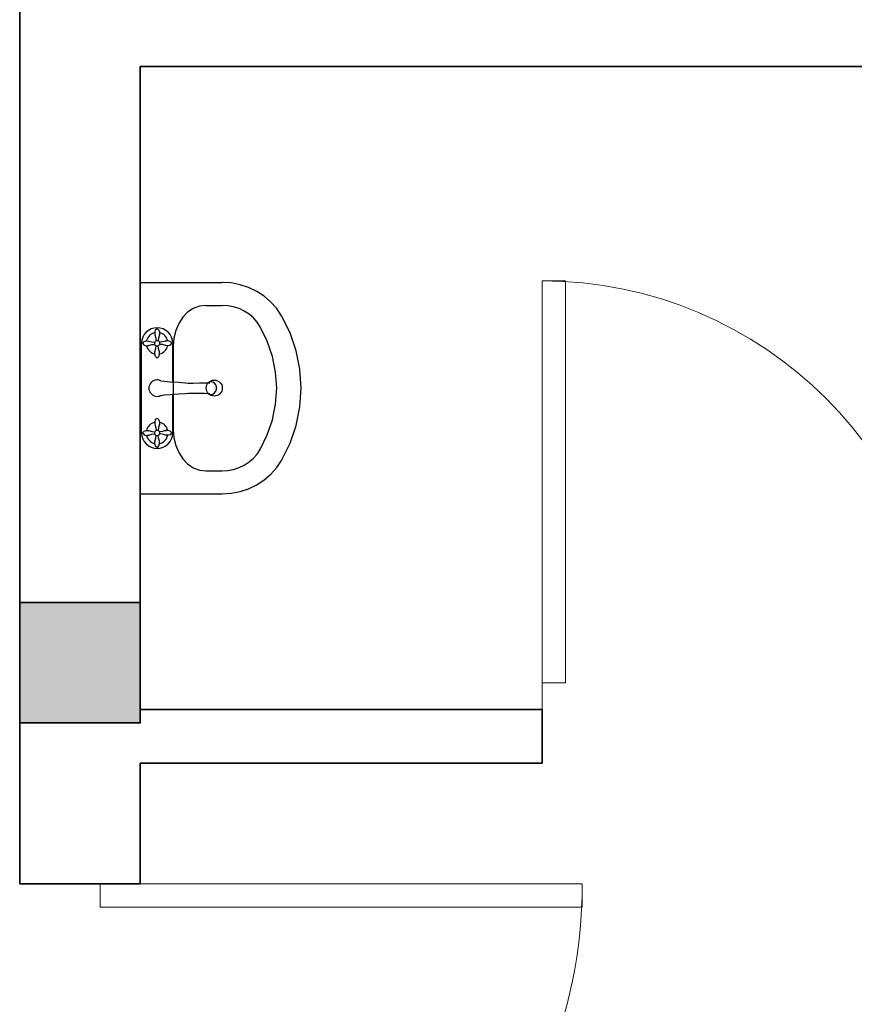
# Model space of a CAD drawing. Units: inches. Extents: x 3321 to 5237, y 11 to 1752.
# Tile 7 of 43: x 3663 to 3725, y 1298 to 1372. Entities that reach past the tile are written whole.
import ezdxf

# ---------------------------------------------------------------- set-up
doc = ezdxf.new("R2010")
doc.units = ezdxf.units.IN
for name, color, linetype, lineweight in [('A-COLS', 1, 'Continuous', 35), ('A-DOOR', 4, 'Continuous', 18), ('A-WALL', 7, 'Continuous', 35), ('Сантехника', 7, 'Continuous', 18)]:
    doc.layers.add(name, color=color, linetype=linetype, lineweight=lineweight)
doc.layers.add('SANTEH', color=7, linetype='Continuous')

# ---------------------------------------------------------------- blocks, each defined once
blk = doc.blocks.new('*U3')
for p, q in [((0, 0), (0, -6)), ((36, 0), (36, -6))]:
    blk.add_line(p, q)
blk.add_lwpolyline([(0, 0), (0, 36), (1.75, 36), (1.75, 0)], close=True)
blk.add_arc((0, 0), 36, 0, 90)
blk = doc.blocks.new('*U6')
for p, q in [((-30, 0), (-30, 6)), ((0, 0), (0, 6))]:
    blk.add_line(p, q)
blk.add_lwpolyline([(0, 0), (0, -30), (-1.75, -30), (-1.75, 0)], close=True)
blk.add_arc((0, 0), 30, 180, 270)
blk = doc.blocks.new('Basin 01_71')
at = {"layer": 'SANTEH'}
for p, q in [((0, 350), (0, 171.8)), ((460, 350), (0, 350)), ((130.2, 343.2), (128.5, 341.7)), ((130.2, 343.2), (128.5, 341.7)), ((130.2, 343.2), (128.5, 341.7)), ((130.2, 343.2), (128.5, 341.7)), ((130.2, 343.2), (128.5, 341.7)), ((130.2, 343.2), (128.5, 341.7)), ((132.5, 345.3), (130.2, 343.2)), ((132.5, 345.3), (130.2, 343.2)), ((132.5, 345.3), (130.2, 343.2)), ((132.5, 345.3), (130.2, 343.2)), ((132.5, 345.3), (130.2, 343.2)), ((132.5, 345.3), (130.2, 343.2)), ((132.5, 346.9), (327.5, 346.9)), ((132.5, 345.3), (134.7, 343.2)), ((132.5, 345.3), (134.7, 343.2)), ((132.5, 345.3), (134.7, 343.2)), ((132.5, 345.3), (134.7, 343.2)), ((132.5, 345.3), (134.7, 343.2)), ((132.5, 345.3), (134.7, 343.2)), ((134.7, 343.2), (136.4, 341.7)), ((134.7, 343.2), (136.4, 341.7)), ((134.7, 343.2), (136.4, 341.7)), ((134.7, 343.2), (136.4, 341.7)), ((134.7, 343.2), (136.4, 341.7)), ((134.7, 343.2), (136.4, 341.7)), ((325.2, 343.2), (323.5, 341.7)), ((325.2, 343.2), (323.5, 341.7)), ((325.2, 343.2), (323.5, 341.7)), ((325.2, 343.2), (323.5, 341.7)), ((325.2, 343.2), (323.5, 341.7)), ((325.2, 343.2), (323.5, 341.7)), ((327.5, 345.3), (325.2, 343.2)), ((327.5, 345.3), (325.2, 343.2)), ((327.5, 345.3), (325.2, 343.2)), ((327.5, 345.3), (325.2, 343.2)), ((327.5, 345.3), (325.2, 343.2)), ((327.5, 345.3), (325.2, 343.2)), ((327.5, 345.3), (329.7, 343.2)), ((327.5, 345.3), (329.7, 343.2)), ((327.5, 345.3), (329.7, 343.2)), ((327.5, 345.3), (329.7, 343.2)), ((327.5, 345.3), (329.7, 343.2)), ((327.5, 345.3), (329.7, 343.2)), ((329.7, 343.2), (331.4, 341.7)), ((329.7, 343.2), (331.4, 341.7)), ((329.7, 343.2), (331.4, 341.7)), ((329.7, 343.2), (331.4, 341.7)), ((329.7, 343.2), (331.4, 341.7)), ((329.7, 343.2), (331.4, 341.7)), ((460, 350), (460, 171.8)), ((128.5, 341.7), (127.2, 337.2)), ((128.5, 341.7), (127.2, 337.2)), ((128.5, 341.7), (127.2, 337.2)), ((128.5, 341.7), (127.2, 337.2)), ((128.5, 341.7), (127.2, 337.2)), ((128.5, 341.7), (127.2, 337.2)), ((127.2, 337.2), (127.5, 332.3)), ((127.2, 337.2), (127.5, 332.3)), ((127.2, 337.2), (127.5, 332.3)), ((127.2, 337.2), (127.5, 332.3)), ((127.2, 337.2), (127.5, 332.3)), ((127.2, 337.2), (127.5, 332.3)), ((127.5, 332.3), (128.4, 332)), ((127.5, 332.3), (128.4, 332)), ((127.5, 332.3), (128.4, 332)), ((127.5, 332.3), (128.4, 332)), ((127.5, 332.3), (128.4, 332)), ((127.5, 332.3), (128.4, 332)), ((128.4, 332), (127.6, 331.5)), ((128.4, 332), (127.6, 331.5)), ((128.4, 332), (127.6, 331.5)), ((128.4, 332), (127.6, 331.5)), ((128.4, 332), (127.6, 331.5)), ((128.4, 332), (127.6, 331.5)), ((127.6, 331.5), (129.6, 324.7)), ((127.6, 331.5), (129.6, 324.7)), ((127.6, 331.5), (129.6, 324.7)), ((127.6, 331.5), (129.6, 324.7)), ((127.6, 331.5), (129.6, 324.7)), ((127.6, 331.5), (129.6, 324.7)), ((129.6, 324.7), (130.2, 318.4)), ((129.6, 324.7), (130.2, 318.4)), ((129.6, 324.7), (130.2, 318.4)), ((129.6, 324.7), (130.2, 318.4)), ((129.6, 324.7), (130.2, 318.4)), ((129.6, 324.7), (130.2, 318.4)), ((135.4, 324.7), (134.8, 318.4)), ((135.4, 324.7), (134.8, 318.4)), ((135.4, 324.7), (134.8, 318.4)), ((135.4, 324.7), (134.8, 318.4)), ((135.4, 324.7), (134.8, 318.4)), ((135.4, 324.7), (134.8, 318.4)), ((137.4, 331.5), (135.4, 324.7)), ((137.4, 331.5), (135.4, 324.7)), ((137.4, 331.5), (135.4, 324.7)), ((137.4, 331.5), (135.4, 324.7)), ((137.4, 331.5), (135.4, 324.7)), ((137.4, 331.5), (135.4, 324.7)), ((136.4, 341.7), (137.7, 337.2)), ((136.4, 341.7), (137.7, 337.2)), ((136.4, 341.7), (137.7, 337.2)), ((136.4, 341.7), (137.7, 337.2)), ((136.4, 341.7), (137.7, 337.2)), ((136.4, 341.7), (137.7, 337.2)), ((137.4, 332.3), (136.6, 332)), ((137.4, 332.3), (136.6, 332)), ((137.4, 332.3), (136.6, 332)), ((137.4, 332.3), (136.6, 332)), ((137.4, 332.3), (136.6, 332)), ((137.4, 332.3), (136.6, 332)), ((136.6, 332), (137.4, 331.5)), ((136.6, 332), (137.4, 331.5)), ((136.6, 332), (137.4, 331.5)), ((136.6, 332), (137.4, 331.5)), ((136.6, 332), (137.4, 331.5)), ((136.6, 332), (137.4, 331.5)), ((137.7, 337.2), (137.4, 332.3)), ((137.7, 337.2), (137.4, 332.3)), ((137.7, 337.2), (137.4, 332.3)), ((137.7, 337.2), (137.4, 332.3)), ((137.7, 337.2), (137.4, 332.3)), ((137.7, 337.2), (137.4, 332.3)), ((323.5, 341.7), (322.2, 337.2)), ((323.5, 341.7), (322.2, 337.2)), ((323.5, 341.7), (322.2, 337.2)), ((323.5, 341.7), (322.2, 337.2)), ((323.5, 341.7), (322.2, 337.2)), ((323.5, 341.7), (322.2, 337.2)), ((322.2, 337.2), (322.5, 332.3)), ((322.2, 337.2), (322.5, 332.3)), ((322.2, 337.2), (322.5, 332.3)), ((322.2, 337.2), (322.5, 332.3)), ((322.2, 337.2), (322.5, 332.3)), ((322.2, 337.2), (322.5, 332.3)), ((322.5, 332.3), (323.4, 332)), ((322.5, 332.3), (323.4, 332)), ((322.5, 332.3), (323.4, 332)), ((322.5, 332.3), (323.4, 332)), ((322.5, 332.3), (323.4, 332)), ((322.5, 332.3), (323.4, 332)), ((323.4, 332), (322.6, 331.5)), ((323.4, 332), (322.6, 331.5)), ((323.4, 332), (322.6, 331.5)), ((323.4, 332), (322.6, 331.5)), ((323.4, 332), (322.6, 331.5)), ((323.4, 332), (322.6, 331.5)), ((322.6, 331.5), (324.6, 324.7)), ((322.6, 331.5), (324.6, 324.7)), ((322.6, 331.5), (324.6, 324.7)), ((322.6, 331.5), (324.6, 324.7)), ((322.6, 331.5), (324.6, 324.7)), ((322.6, 331.5), (324.6, 324.7)), ((324.6, 324.7), (325.2, 318.4)), ((324.6, 324.7), (325.2, 318.4)), ((324.6, 324.7), (325.2, 318.4)), ((324.6, 324.7), (325.2, 318.4)), ((324.6, 324.7), (325.2, 318.4)), ((324.6, 324.7), (325.2, 318.4)), ((330.4, 324.7), (329.8, 318.4)), ((330.4, 324.7), (329.8, 318.4)), ((330.4, 324.7), (329.8, 318.4)), ((330.4, 324.7), (329.8, 318.4)), ((330.4, 324.7), (329.8, 318.4)), ((330.4, 324.7), (329.8, 318.4)), ((332.4, 331.5), (330.4, 324.7)), ((332.4, 331.5), (330.4, 324.7)), ((332.4, 331.5), (330.4, 324.7)), ((332.4, 331.5), (330.4, 324.7)), ((332.4, 331.5), (330.4, 324.7)), ((332.4, 331.5), (330.4, 324.7)), ((331.4, 341.7), (332.7, 337.2)), ((331.4, 341.7), (332.7, 337.2)), ((331.4, 341.7), (332.7, 337.2)), ((331.4, 341.7), (332.7, 337.2)), ((331.4, 341.7), (332.7, 337.2)), ((331.4, 341.7), (332.7, 337.2)), ((332.4, 332.3), (331.6, 332)), ((332.4, 332.3), (331.6, 332)), ((332.4, 332.3), (331.6, 332)), ((332.4, 332.3), (331.6, 332)), ((332.4, 332.3), (331.6, 332)), ((332.4, 332.3), (331.6, 332)), ((331.6, 332), (332.4, 331.5)), ((331.6, 332), (332.4, 331.5)), ((331.6, 332), (332.4, 331.5)), ((331.6, 332), (332.4, 331.5)), ((331.6, 332), (332.4, 331.5)), ((331.6, 332), (332.4, 331.5)), ((332.7, 337.2), (332.4, 332.3)), ((332.7, 337.2), (332.4, 332.3)), ((332.7, 337.2), (332.4, 332.3)), ((332.7, 337.2), (332.4, 332.3)), ((332.7, 337.2), (332.4, 332.3)), ((332.7, 337.2), (332.4, 332.3)), ((100.4, 313.2), (102.5, 315.4)), ((100.4, 313.2), (102.5, 315.4)), ((100.4, 313.2), (102.5, 315.4)), ((100.4, 313.2), (102.5, 315.4)), ((100.4, 313.2), (102.5, 315.4)), ((100.4, 313.2), (102.5, 315.4)), ((100.4, 313.2), (102.5, 310.9)), ((100.4, 313.2), (102.5, 310.9)), ((100.4, 313.2), (102.5, 310.9)), ((100.4, 313.2), (102.5, 310.9)), ((100.4, 313.2), (102.5, 310.9)), ((100.4, 313.2), (102.5, 310.9)), ((102.5, 315.4), (104, 317.1)), ((102.5, 315.4), (104, 317.1)), ((102.5, 315.4), (104, 317.1)), ((102.5, 315.4), (104, 317.1)), ((102.5, 315.4), (104, 317.1)), ((102.5, 315.4), (104, 317.1)), ((102.5, 310.9), (104, 309.2)), ((102.5, 310.9), (104, 309.2)), ((102.5, 310.9), (104, 309.2)), ((102.5, 310.9), (104, 309.2)), ((102.5, 310.9), (104, 309.2)), ((102.5, 310.9), (104, 309.2)), ((104, 317.1), (108.5, 318.4)), ((104, 317.1), (108.5, 318.4)), ((104, 317.1), (108.5, 318.4)), ((104, 317.1), (108.5, 318.4)), ((104, 317.1), (108.5, 318.4)), ((104, 317.1), (108.5, 318.4)), ((104, 309.2), (108.5, 307.9)), ((104, 309.2), (108.5, 307.9)), ((104, 309.2), (108.5, 307.9)), ((104, 309.2), (108.5, 307.9)), ((104, 309.2), (108.5, 307.9)), ((104, 309.2), (108.5, 307.9)), ((108.5, 318.4), (113.4, 318.1)), ((108.5, 318.4), (113.4, 318.1)), ((108.5, 318.4), (113.4, 318.1)), ((108.5, 318.4), (113.4, 318.1)), ((108.5, 318.4), (113.4, 318.1)), ((108.5, 318.4), (113.4, 318.1)), ((108.5, 307.9), (113.4, 308.2)), ((108.5, 307.9), (113.4, 308.2)), ((108.5, 307.9), (113.4, 308.2)), ((108.5, 307.9), (113.4, 308.2)), ((108.5, 307.9), (113.4, 308.2)), ((108.5, 307.9), (113.4, 308.2)), ((113.4, 318.1), (113.7, 317.3)), ((113.4, 318.1), (113.7, 317.3)), ((113.4, 318.1), (113.7, 317.3)), ((113.4, 318.1), (113.7, 317.3)), ((113.4, 318.1), (113.7, 317.3)), ((113.4, 318.1), (113.7, 317.3)), ((113.4, 308.2), (113.7, 309.1)), ((113.4, 308.2), (113.7, 309.1)), ((113.4, 308.2), (113.7, 309.1)), ((113.4, 308.2), (113.7, 309.1)), ((113.4, 308.2), (113.7, 309.1)), ((113.4, 308.2), (113.7, 309.1)), ((113.7, 317.3), (114.2, 318.1)), ((113.7, 317.3), (114.2, 318.1)), ((113.7, 317.3), (114.2, 318.1)), ((113.7, 317.3), (114.2, 318.1)), ((113.7, 317.3), (114.2, 318.1)), ((113.7, 317.3), (114.2, 318.1)), ((113.7, 309.1), (114.2, 308.3)), ((113.7, 309.1), (114.2, 308.3)), ((113.7, 309.1), (114.2, 308.3)), ((113.7, 309.1), (114.2, 308.3)), ((113.7, 309.1), (114.2, 308.3)), ((113.7, 309.1), (114.2, 308.3)), ((114.2, 318.1), (121, 316.1)), ((114.2, 318.1), (121, 316.1)), ((114.2, 318.1), (121, 316.1)), ((114.2, 318.1), (121, 316.1)), ((114.2, 318.1), (121, 316.1)), ((114.2, 318.1), (121, 316.1)), ((114.2, 308.3), (121, 310.3)), ((114.2, 308.3), (121, 310.3)), ((114.2, 308.3), (121, 310.3)), ((114.2, 308.3), (121, 310.3)), ((114.2, 308.3), (121, 310.3)), ((114.2, 308.3), (121, 310.3)), ((121, 316.1), (127.3, 315.5)), ((121, 316.1), (127.3, 315.5)), ((121, 316.1), (127.3, 315.5)), ((121, 316.1), (127.3, 315.5)), ((121, 316.1), (127.3, 315.5)), ((121, 316.1), (127.3, 315.5)), ((121, 310.3), (127.3, 310.9)), ((121, 310.3), (127.3, 310.9)), ((121, 310.3), (127.3, 310.9)), ((121, 310.3), (127.3, 310.9)), ((121, 310.3), (127.3, 310.9)), ((121, 310.3), (127.3, 310.9)), ((127.1, 315.1), (126.8, 313.9)), ((127.1, 315.1), (126.8, 313.9)), ((127.1, 315.1), (126.8, 313.9)), ((127.1, 315.1), (126.8, 313.9)), ((127.1, 315.1), (126.8, 313.9)), ((127.1, 315.1), (126.8, 313.9)), ((126.8, 313.9), (126.8, 312.5)), ((126.8, 313.9), (126.8, 312.5)), ((126.8, 313.9), (126.8, 312.5)), ((126.8, 313.9), (126.8, 312.5)), ((126.8, 313.9), (126.8, 312.5)), ((126.8, 313.9), (126.8, 312.5)), ((126.8, 312.5), (127.1, 311.2)), ((126.8, 312.5), (127.1, 311.2)), ((126.8, 312.5), (127.1, 311.2)), ((126.8, 312.5), (127.1, 311.2)), ((126.8, 312.5), (127.1, 311.2)), ((126.8, 312.5), (127.1, 311.2)), ((127.7, 316.3), (127.1, 315.1)), ((127.7, 316.3), (127.1, 315.1)), ((127.7, 316.3), (127.1, 315.1)), ((127.7, 316.3), (127.1, 315.1)), ((127.7, 316.3), (127.1, 315.1)), ((127.7, 316.3), (127.1, 315.1)), ((127.1, 311.2), (127.7, 310.1)), ((127.1, 311.2), (127.7, 310.1)), ((127.1, 311.2), (127.7, 310.1)), ((127.1, 311.2), (127.7, 310.1)), ((127.1, 311.2), (127.7, 310.1)), ((127.1, 311.2), (127.7, 310.1)), ((127.6, 294.9), (129.6, 301.7)), ((127.6, 294.9), (129.6, 301.7)), ((127.6, 294.9), (129.6, 301.7)), ((127.6, 294.9), (129.6, 301.7)), ((127.6, 294.9), (129.6, 301.7)), ((127.6, 294.9), (129.6, 301.7)), ((128.6, 317.3), (127.7, 316.3)), ((128.6, 317.3), (127.7, 316.3)), ((128.6, 317.3), (127.7, 316.3)), ((128.6, 317.3), (127.7, 316.3)), ((128.6, 317.3), (127.7, 316.3)), ((128.6, 317.3), (127.7, 316.3)), ((127.7, 310.1), (128.6, 309.1)), ((127.7, 310.1), (128.6, 309.1)), ((127.7, 310.1), (128.6, 309.1)), ((127.7, 310.1), (128.6, 309.1)), ((127.7, 310.1), (128.6, 309.1)), ((127.7, 310.1), (128.6, 309.1)), ((129.7, 318.1), (128.6, 317.3)), ((129.7, 318.1), (128.6, 317.3)), ((129.7, 318.1), (128.6, 317.3)), ((129.7, 318.1), (128.6, 317.3)), ((129.7, 318.1), (128.6, 317.3)), ((129.7, 318.1), (128.6, 317.3)), ((128.6, 309.1), (129.7, 308.3)), ((128.6, 309.1), (129.7, 308.3)), ((128.6, 309.1), (129.7, 308.3)), ((128.6, 309.1), (129.7, 308.3)), ((128.6, 309.1), (129.7, 308.3)), ((128.6, 309.1), (129.7, 308.3)), ((129.6, 301.7), (130.2, 308)), ((129.6, 301.7), (130.2, 308)), ((129.6, 301.7), (130.2, 308)), ((129.6, 301.7), (130.2, 308)), ((129.6, 301.7), (130.2, 308)), ((129.6, 301.7), (130.2, 308)), ((130.9, 318.7), (129.7, 318.1)), ((130.9, 318.7), (129.7, 318.1)), ((130.9, 318.7), (129.7, 318.1)), ((130.9, 318.7), (129.7, 318.1)), ((130.9, 318.7), (129.7, 318.1)), ((130.9, 318.7), (129.7, 318.1)), ((129.7, 308.3), (130.9, 307.7)), ((129.7, 308.3), (130.9, 307.7)), ((129.7, 308.3), (130.9, 307.7)), ((129.7, 308.3), (130.9, 307.7)), ((129.7, 308.3), (130.9, 307.7)), ((129.7, 308.3), (130.9, 307.7)), ((132.2, 318.9), (130.9, 318.7)), ((132.2, 318.9), (130.9, 318.7)), ((132.2, 318.9), (130.9, 318.7)), ((132.2, 318.9), (130.9, 318.7)), ((132.2, 318.9), (130.9, 318.7)), ((132.2, 318.9), (130.9, 318.7)), ((130.9, 307.7), (132.2, 307.5)), ((130.9, 307.7), (132.2, 307.5)), ((130.9, 307.7), (132.2, 307.5)), ((130.9, 307.7), (132.2, 307.5)), ((130.9, 307.7), (132.2, 307.5)), ((130.9, 307.7), (132.2, 307.5)), ((133.5, 318.8), (132.2, 318.9)), ((133.5, 318.8), (132.2, 318.9)), ((133.5, 318.8), (132.2, 318.9)), ((133.5, 318.8), (132.2, 318.9)), ((133.5, 318.8), (132.2, 318.9)), ((133.5, 318.8), (132.2, 318.9)), ((132.2, 307.5), (133.5, 307.6)), ((132.2, 307.5), (133.5, 307.6)), ((132.2, 307.5), (133.5, 307.6)), ((132.2, 307.5), (133.5, 307.6)), ((132.2, 307.5), (133.5, 307.6)), ((132.2, 307.5), (133.5, 307.6)), ((134.8, 318.4), (133.5, 318.8)), ((134.8, 318.4), (133.5, 318.8)), ((134.8, 318.4), (133.5, 318.8)), ((134.8, 318.4), (133.5, 318.8)), ((134.8, 318.4), (133.5, 318.8)), ((134.8, 318.4), (133.5, 318.8)), ((133.5, 307.6), (134.8, 308)), ((133.5, 307.6), (134.8, 308)), ((133.5, 307.6), (134.8, 308)), ((133.5, 307.6), (134.8, 308)), ((133.5, 307.6), (134.8, 308)), ((133.5, 307.6), (134.8, 308)), ((135.9, 317.8), (134.8, 318.4)), ((135.9, 317.8), (134.8, 318.4)), ((135.9, 317.8), (134.8, 318.4)), ((135.9, 317.8), (134.8, 318.4)), ((135.9, 317.8), (134.8, 318.4)), ((135.9, 317.8), (134.8, 318.4)), ((134.8, 308), (135.9, 308.6)), ((134.8, 308), (135.9, 308.6)), ((134.8, 308), (135.9, 308.6)), ((134.8, 308), (135.9, 308.6)), ((134.8, 308), (135.9, 308.6)), ((134.8, 308), (135.9, 308.6)), ((135.4, 301.7), (134.8, 308)), ((135.4, 301.7), (134.8, 308)), ((135.4, 301.7), (134.8, 308)), ((135.4, 301.7), (134.8, 308)), ((135.4, 301.7), (134.8, 308)), ((135.4, 301.7), (134.8, 308)), ((137.4, 294.9), (135.4, 301.7)), ((137.4, 294.9), (135.4, 301.7)), ((137.4, 294.9), (135.4, 301.7)), ((137.4, 294.9), (135.4, 301.7)), ((137.4, 294.9), (135.4, 301.7)), ((137.4, 294.9), (135.4, 301.7)), ((136.9, 316.9), (135.9, 317.8)), ((136.9, 316.9), (135.9, 317.8)), ((136.9, 316.9), (135.9, 317.8)), ((136.9, 316.9), (135.9, 317.8)), ((136.9, 316.9), (135.9, 317.8)), ((136.9, 316.9), (135.9, 317.8)), ((135.9, 308.6), (136.9, 309.5)), ((135.9, 308.6), (136.9, 309.5)), ((135.9, 308.6), (136.9, 309.5)), ((135.9, 308.6), (136.9, 309.5)), ((135.9, 308.6), (136.9, 309.5)), ((135.9, 308.6), (136.9, 309.5)), ((137.6, 315.8), (136.9, 316.9)), ((137.6, 315.8), (136.9, 316.9)), ((137.6, 315.8), (136.9, 316.9)), ((137.6, 315.8), (136.9, 316.9)), ((137.6, 315.8), (136.9, 316.9)), ((137.6, 315.8), (136.9, 316.9)), ((136.9, 309.5), (137.6, 310.6)), ((136.9, 309.5), (137.6, 310.6)), ((136.9, 309.5), (137.6, 310.6)), ((136.9, 309.5), (137.6, 310.6)), ((136.9, 309.5), (137.6, 310.6)), ((136.9, 309.5), (137.6, 310.6)), ((138, 314.5), (137.6, 315.8)), ((138, 314.5), (137.6, 315.8)), ((138, 314.5), (137.6, 315.8)), ((138, 314.5), (137.6, 315.8)), ((138, 314.5), (137.6, 315.8)), ((138, 314.5), (137.6, 315.8)), ((137.6, 310.6), (138, 311.9)), ((137.6, 310.6), (138, 311.9)), ((137.6, 310.6), (138, 311.9)), ((137.6, 310.6), (138, 311.9)), ((137.6, 310.6), (138, 311.9)), ((137.6, 310.6), (138, 311.9)), ((144, 316.1), (137.7, 315.5)), ((144, 316.1), (137.7, 315.5)), ((144, 316.1), (137.7, 315.5)), ((144, 316.1), (137.7, 315.5)), ((144, 316.1), (137.7, 315.5)), ((144, 316.1), (137.7, 315.5)), ((144, 310.3), (137.7, 310.9)), ((144, 310.3), (137.7, 310.9)), ((144, 310.3), (137.7, 310.9)), ((144, 310.3), (137.7, 310.9)), ((144, 310.3), (137.7, 310.9)), ((144, 310.3), (137.7, 310.9)), ((138.2, 313.2), (138, 314.5)), ((138.2, 313.2), (138, 314.5)), ((138.2, 313.2), (138, 314.5)), ((138.2, 313.2), (138, 314.5)), ((138.2, 313.2), (138, 314.5)), ((138.2, 313.2), (138, 314.5)), ((138, 311.9), (138.2, 313.2)), ((138, 311.9), (138.2, 313.2)), ((138, 311.9), (138.2, 313.2)), ((138, 311.9), (138.2, 313.2)), ((138, 311.9), (138.2, 313.2)), ((138, 311.9), (138.2, 313.2)), ((150.8, 318.1), (144, 316.1)), ((150.8, 318.1), (144, 316.1)), ((150.8, 318.1), (144, 316.1)), ((150.8, 318.1), (144, 316.1)), ((150.8, 318.1), (144, 316.1)), ((150.8, 318.1), (144, 316.1)), ((150.8, 308.3), (144, 310.3)), ((150.8, 308.3), (144, 310.3)), ((150.8, 308.3), (144, 310.3)), ((150.8, 308.3), (144, 310.3)), ((150.8, 308.3), (144, 310.3)), ((150.8, 308.3), (144, 310.3)), ((151.3, 317.3), (150.8, 318.1)), ((151.3, 317.3), (150.8, 318.1)), ((151.3, 317.3), (150.8, 318.1)), ((151.3, 317.3), (150.8, 318.1)), ((151.3, 317.3), (150.8, 318.1)), ((151.3, 317.3), (150.8, 318.1)), ((151.3, 309.1), (150.8, 308.3)), ((151.3, 309.1), (150.8, 308.3)), ((151.3, 309.1), (150.8, 308.3)), ((151.3, 309.1), (150.8, 308.3)), ((151.3, 309.1), (150.8, 308.3)), ((151.3, 309.1), (150.8, 308.3)), ((151.6, 318.1), (151.3, 317.3)), ((151.6, 318.1), (151.3, 317.3)), ((151.6, 318.1), (151.3, 317.3)), ((151.6, 318.1), (151.3, 317.3)), ((151.6, 318.1), (151.3, 317.3)), ((151.6, 318.1), (151.3, 317.3)), ((151.6, 308.3), (151.3, 309.1)), ((151.6, 308.3), (151.3, 309.1)), ((151.6, 308.3), (151.3, 309.1)), ((151.6, 308.3), (151.3, 309.1)), ((151.6, 308.3), (151.3, 309.1)), ((151.6, 308.3), (151.3, 309.1)), ((156.5, 318.4), (151.6, 318.1)), ((156.5, 318.4), (151.6, 318.1)), ((156.5, 318.4), (151.6, 318.1)), ((156.5, 318.4), (151.6, 318.1)), ((156.5, 318.4), (151.6, 318.1)), ((156.5, 318.4), (151.6, 318.1)), ((156.5, 308), (151.6, 308.3)), ((156.5, 308), (151.6, 308.3)), ((156.5, 308), (151.6, 308.3)), ((156.5, 308), (151.6, 308.3)), ((156.5, 308), (151.6, 308.3)), ((156.5, 308), (151.6, 308.3)), ((161, 317.2), (156.5, 318.4)), ((161, 317.2), (156.5, 318.4)), ((161, 317.2), (156.5, 318.4)), ((161, 317.2), (156.5, 318.4)), ((161, 317.2), (156.5, 318.4)), ((161, 317.2), (156.5, 318.4)), ((161, 309.2), (156.5, 308)), ((161, 309.2), (156.5, 308)), ((161, 309.2), (156.5, 308)), ((161, 309.2), (156.5, 308)), ((161, 309.2), (156.5, 308)), ((161, 309.2), (156.5, 308)), ((162.5, 315.4), (161, 317.2)), ((162.5, 315.4), (161, 317.2)), ((162.5, 315.4), (161, 317.2)), ((162.5, 315.4), (161, 317.2)), ((162.5, 315.4), (161, 317.2)), ((162.5, 315.4), (161, 317.2)), ((162.5, 311), (161, 309.2)), ((162.5, 311), (161, 309.2)), ((162.5, 311), (161, 309.2)), ((162.5, 311), (161, 309.2)), ((162.5, 311), (161, 309.2)), ((162.5, 311), (161, 309.2)), ((164.6, 313.2), (162.5, 315.4)), ((164.6, 313.2), (162.5, 315.4)), ((164.6, 313.2), (162.5, 315.4)), ((164.6, 313.2), (162.5, 315.4)), ((164.6, 313.2), (162.5, 315.4)), ((164.6, 313.2), (162.5, 315.4)), ((164.6, 313.2), (162.5, 311)), ((164.6, 313.2), (162.5, 311)), ((164.6, 313.2), (162.5, 311)), ((164.6, 313.2), (162.5, 311)), ((164.6, 313.2), (162.5, 311)), ((164.6, 313.2), (162.5, 311)), ((213.9, 305.1), (215, 298)), ((246.1, 305.1), (245, 298)), ((295.4, 313.2), (297.5, 315.4)), ((295.4, 313.2), (297.5, 315.4)), ((295.4, 313.2), (297.5, 315.4)), ((295.4, 313.2), (297.5, 315.4)), ((295.4, 313.2), (297.5, 315.4)), ((295.4, 313.2), (297.5, 315.4)), ((295.4, 313.2), (297.5, 310.9)), ((295.4, 313.2), (297.5, 310.9)), ((295.4, 313.2), (297.5, 310.9)), ((295.4, 313.2), (297.5, 310.9)), ((295.4, 313.2), (297.5, 310.9)), ((295.4, 313.2), (297.5, 310.9)), ((297.5, 315.4), (299, 317.1)), ((297.5, 315.4), (299, 317.1)), ((297.5, 315.4), (299, 317.1)), ((297.5, 315.4), (299, 317.1)), ((297.5, 315.4), (299, 317.1)), ((297.5, 315.4), (299, 317.1)), ((297.5, 310.9), (299, 309.2)), ((297.5, 310.9), (299, 309.2)), ((297.5, 310.9), (299, 309.2)), ((297.5, 310.9), (299, 309.2)), ((297.5, 310.9), (299, 309.2)), ((297.5, 310.9), (299, 309.2)), ((299, 317.1), (303.5, 318.4)), ((299, 317.1), (303.5, 318.4)), ((299, 317.1), (303.5, 318.4)), ((299, 317.1), (303.5, 318.4)), ((299, 317.1), (303.5, 318.4)), ((299, 317.1), (303.5, 318.4)), ((299, 309.2), (303.5, 307.9)), ((299, 309.2), (303.5, 307.9)), ((299, 309.2), (303.5, 307.9)), ((299, 309.2), (303.5, 307.9)), ((299, 309.2), (303.5, 307.9)), ((299, 309.2), (303.5, 307.9)), ((303.5, 318.4), (308.4, 318.1)), ((303.5, 318.4), (308.4, 318.1)), ((303.5, 318.4), (308.4, 318.1)), ((303.5, 318.4), (308.4, 318.1)), ((303.5, 318.4), (308.4, 318.1)), ((303.5, 318.4), (308.4, 318.1)), ((303.5, 307.9), (308.4, 308.2)), ((303.5, 307.9), (308.4, 308.2)), ((303.5, 307.9), (308.4, 308.2)), ((303.5, 307.9), (308.4, 308.2)), ((303.5, 307.9), (308.4, 308.2)), ((303.5, 307.9), (308.4, 308.2)), ((308.4, 318.1), (308.7, 317.3)), ((308.4, 318.1), (308.7, 317.3)), ((308.4, 318.1), (308.7, 317.3)), ((308.4, 318.1), (308.7, 317.3)), ((308.4, 318.1), (308.7, 317.3)), ((308.4, 318.1), (308.7, 317.3)), ((308.4, 308.2), (308.7, 309.1)), ((308.4, 308.2), (308.7, 309.1)), ((308.4, 308.2), (308.7, 309.1)), ((308.4, 308.2), (308.7, 309.1)), ((308.4, 308.2), (308.7, 309.1)), ((308.4, 308.2), (308.7, 309.1)), ((308.7, 317.3), (309.2, 318.1)), ((308.7, 317.3), (309.2, 318.1)), ((308.7, 317.3), (309.2, 318.1)), ((308.7, 317.3), (309.2, 318.1)), ((308.7, 317.3), (309.2, 318.1)), ((308.7, 317.3), (309.2, 318.1)), ((308.7, 309.1), (309.2, 308.3)), ((308.7, 309.1), (309.2, 308.3)), ((308.7, 309.1), (309.2, 308.3)), ((308.7, 309.1), (309.2, 308.3)), ((308.7, 309.1), (309.2, 308.3)), ((308.7, 309.1), (309.2, 308.3)), ((309.2, 318.1), (316, 316.1)), ((309.2, 318.1), (316, 316.1)), ((309.2, 318.1), (316, 316.1)), ((309.2, 318.1), (316, 316.1)), ((309.2, 318.1), (316, 316.1)), ((309.2, 318.1), (316, 316.1)), ((309.2, 308.3), (316, 310.3)), ((309.2, 308.3), (316, 310.3)), ((309.2, 308.3), (316, 310.3)), ((309.2, 308.3), (316, 310.3)), ((309.2, 308.3), (316, 310.3)), ((309.2, 308.3), (316, 310.3)), ((316, 316.1), (322.3, 315.5)), ((316, 316.1), (322.3, 315.5)), ((316, 316.1), (322.3, 315.5)), ((316, 316.1), (322.3, 315.5)), ((316, 316.1), (322.3, 315.5)), ((316, 316.1), (322.3, 315.5)), ((316, 310.3), (322.3, 310.9)), ((316, 310.3), (322.3, 310.9)), ((316, 310.3), (322.3, 310.9)), ((316, 310.3), (322.3, 310.9)), ((316, 310.3), (322.3, 310.9)), ((316, 310.3), (322.3, 310.9)), ((322.1, 315.1), (321.8, 313.9)), ((322.1, 315.1), (321.8, 313.9)), ((322.1, 315.1), (321.8, 313.9)), ((322.1, 315.1), (321.8, 313.9)), ((322.1, 315.1), (321.8, 313.9)), ((322.1, 315.1), (321.8, 313.9)), ((321.8, 313.9), (321.8, 312.5)), ((321.8, 313.9), (321.8, 312.5)), ((321.8, 313.9), (321.8, 312.5)), ((321.8, 313.9), (321.8, 312.5)), ((321.8, 313.9), (321.8, 312.5)), ((321.8, 313.9), (321.8, 312.5)), ((321.8, 312.5), (322.1, 311.2)), ((321.8, 312.5), (322.1, 311.2)), ((321.8, 312.5), (322.1, 311.2)), ((321.8, 312.5), (322.1, 311.2)), ((321.8, 312.5), (322.1, 311.2)), ((321.8, 312.5), (322.1, 311.2)), ((322.7, 316.3), (322.1, 315.1)), ((322.7, 316.3), (322.1, 315.1)), ((322.7, 316.3), (322.1, 315.1)), ((322.7, 316.3), (322.1, 315.1)), ((322.7, 316.3), (322.1, 315.1)), ((322.7, 316.3), (322.1, 315.1)), ((322.1, 311.2), (322.7, 310.1)), ((322.1, 311.2), (322.7, 310.1)), ((322.1, 311.2), (322.7, 310.1)), ((322.1, 311.2), (322.7, 310.1)), ((322.1, 311.2), (322.7, 310.1)), ((322.1, 311.2), (322.7, 310.1)), ((322.6, 294.9), (324.6, 301.7)), ((322.6, 294.9), (324.6, 301.7)), ((322.6, 294.9), (324.6, 301.7)), ((322.6, 294.9), (324.6, 301.7)), ((322.6, 294.9), (324.6, 301.7)), ((322.6, 294.9), (324.6, 301.7)), ((323.6, 317.3), (322.7, 316.3)), ((323.6, 317.3), (322.7, 316.3)), ((323.6, 317.3), (322.7, 316.3)), ((323.6, 317.3), (322.7, 316.3)), ((323.6, 317.3), (322.7, 316.3)), ((323.6, 317.3), (322.7, 316.3)), ((322.7, 310.1), (323.6, 309.1)), ((322.7, 310.1), (323.6, 309.1)), ((322.7, 310.1), (323.6, 309.1)), ((322.7, 310.1), (323.6, 309.1)), ((322.7, 310.1), (323.6, 309.1)), ((322.7, 310.1), (323.6, 309.1)), ((324.7, 318.1), (323.6, 317.3)), ((324.7, 318.1), (323.6, 317.3)), ((324.7, 318.1), (323.6, 317.3)), ((324.7, 318.1), (323.6, 317.3)), ((324.7, 318.1), (323.6, 317.3)), ((324.7, 318.1), (323.6, 317.3)), ((323.6, 309.1), (324.7, 308.3)), ((323.6, 309.1), (324.7, 308.3)), ((323.6, 309.1), (324.7, 308.3)), ((323.6, 309.1), (324.7, 308.3)), ((323.6, 309.1), (324.7, 308.3)), ((323.6, 309.1), (324.7, 308.3)), ((324.6, 301.7), (325.2, 308)), ((324.6, 301.7), (325.2, 308)), ((324.6, 301.7), (325.2, 308)), ((324.6, 301.7), (325.2, 308)), ((324.6, 301.7), (325.2, 308)), ((324.6, 301.7), (325.2, 308)), ((325.9, 318.7), (324.7, 318.1)), ((325.9, 318.7), (324.7, 318.1)), ((325.9, 318.7), (324.7, 318.1)), ((325.9, 318.7), (324.7, 318.1)), ((325.9, 318.7), (324.7, 318.1)), ((325.9, 318.7), (324.7, 318.1)), ((324.7, 308.3), (325.9, 307.7)), ((324.7, 308.3), (325.9, 307.7)), ((324.7, 308.3), (325.9, 307.7)), ((324.7, 308.3), (325.9, 307.7)), ((324.7, 308.3), (325.9, 307.7)), ((324.7, 308.3), (325.9, 307.7)), ((327.2, 318.9), (325.9, 318.7)), ((327.2, 318.9), (325.9, 318.7)), ((327.2, 318.9), (325.9, 318.7)), ((327.2, 318.9), (325.9, 318.7)), ((327.2, 318.9), (325.9, 318.7)), ((327.2, 318.9), (325.9, 318.7)), ((325.9, 307.7), (327.2, 307.5)), ((325.9, 307.7), (327.2, 307.5)), ((325.9, 307.7), (327.2, 307.5)), ((325.9, 307.7), (327.2, 307.5)), ((325.9, 307.7), (327.2, 307.5)), ((325.9, 307.7), (327.2, 307.5)), ((328.5, 318.8), (327.2, 318.9)), ((328.5, 318.8), (327.2, 318.9)), ((328.5, 318.8), (327.2, 318.9)), ((328.5, 318.8), (327.2, 318.9)), ((328.5, 318.8), (327.2, 318.9)), ((328.5, 318.8), (327.2, 318.9)), ((327.2, 307.5), (328.5, 307.6)), ((327.2, 307.5), (328.5, 307.6)), ((327.2, 307.5), (328.5, 307.6)), ((327.2, 307.5), (328.5, 307.6)), ((327.2, 307.5), (328.5, 307.6)), ((327.2, 307.5), (328.5, 307.6)), ((329.8, 318.4), (328.5, 318.8)), ((329.8, 318.4), (328.5, 318.8)), ((329.8, 318.4), (328.5, 318.8)), ((329.8, 318.4), (328.5, 318.8)), ((329.8, 318.4), (328.5, 318.8)), ((329.8, 318.4), (328.5, 318.8)), ((328.5, 307.6), (329.8, 308)), ((328.5, 307.6), (329.8, 308)), ((328.5, 307.6), (329.8, 308)), ((328.5, 307.6), (329.8, 308)), ((328.5, 307.6), (329.8, 308)), ((328.5, 307.6), (329.8, 308)), ((330.9, 317.8), (329.8, 318.4)), ((330.9, 317.8), (329.8, 318.4)), ((330.9, 317.8), (329.8, 318.4)), ((330.9, 317.8), (329.8, 318.4)), ((330.9, 317.8), (329.8, 318.4)), ((330.9, 317.8), (329.8, 318.4)), ((329.8, 308), (330.9, 308.6)), ((329.8, 308), (330.9, 308.6)), ((329.8, 308), (330.9, 308.6)), ((329.8, 308), (330.9, 308.6)), ((329.8, 308), (330.9, 308.6)), ((329.8, 308), (330.9, 308.6)), ((330.4, 301.7), (329.8, 308)), ((330.4, 301.7), (329.8, 308)), ((330.4, 301.7), (329.8, 308)), ((330.4, 301.7), (329.8, 308)), ((330.4, 301.7), (329.8, 308)), ((330.4, 301.7), (329.8, 308)), ((332.4, 294.9), (330.4, 301.7)), ((332.4, 294.9), (330.4, 301.7)), ((332.4, 294.9), (330.4, 301.7)), ((332.4, 294.9), (330.4, 301.7)), ((332.4, 294.9), (330.4, 301.7)), ((332.4, 294.9), (330.4, 301.7)), ((331.9, 316.9), (330.9, 317.8)), ((331.9, 316.9), (330.9, 317.8)), ((331.9, 316.9), (330.9, 317.8)), ((331.9, 316.9), (330.9, 317.8)), ((331.9, 316.9), (330.9, 317.8)), ((331.9, 316.9), (330.9, 317.8)), ((330.9, 308.6), (331.9, 309.5)), ((330.9, 308.6), (331.9, 309.5)), ((330.9, 308.6), (331.9, 309.5)), ((330.9, 308.6), (331.9, 309.5)), ((330.9, 308.6), (331.9, 309.5)), ((330.9, 308.6), (331.9, 309.5)), ((332.6, 315.8), (331.9, 316.9)), ((332.6, 315.8), (331.9, 316.9)), ((332.6, 315.8), (331.9, 316.9)), ((332.6, 315.8), (331.9, 316.9)), ((332.6, 315.8), (331.9, 316.9)), ((332.6, 315.8), (331.9, 316.9)), ((331.9, 309.5), (332.6, 310.6)), ((331.9, 309.5), (332.6, 310.6)), ((331.9, 309.5), (332.6, 310.6)), ((331.9, 309.5), (332.6, 310.6)), ((331.9, 309.5), (332.6, 310.6)), ((331.9, 309.5), (332.6, 310.6)), ((333, 314.5), (332.6, 315.8)), ((333, 314.5), (332.6, 315.8)), ((333, 314.5), (332.6, 315.8)), ((333, 314.5), (332.6, 315.8)), ((333, 314.5), (332.6, 315.8)), ((333, 314.5), (332.6, 315.8)), ((332.6, 310.6), (333, 311.9)), ((332.6, 310.6), (333, 311.9)), ((332.6, 310.6), (333, 311.9)), ((332.6, 310.6), (333, 311.9)), ((332.6, 310.6), (333, 311.9)), ((332.6, 310.6), (333, 311.9)), ((339, 316.1), (332.7, 315.5)), ((339, 316.1), (332.7, 315.5)), ((339, 316.1), (332.7, 315.5)), ((339, 316.1), (332.7, 315.5)), ((339, 316.1), (332.7, 315.5)), ((339, 316.1), (332.7, 315.5)), ((339, 310.3), (332.7, 310.9)), ((339, 310.3), (332.7, 310.9)), ((339, 310.3), (332.7, 310.9)), ((339, 310.3), (332.7, 310.9)), ((339, 310.3), (332.7, 310.9)), ((339, 310.3), (332.7, 310.9)), ((333.2, 313.2), (333, 314.5)), ((333.2, 313.2), (333, 314.5)), ((333.2, 313.2), (333, 314.5)), ((333.2, 313.2), (333, 314.5)), ((333.2, 313.2), (333, 314.5)), ((333.2, 313.2), (333, 314.5)), ((333, 311.9), (333.2, 313.2)), ((333, 311.9), (333.2, 313.2)), ((333, 311.9), (333.2, 313.2)), ((333, 311.9), (333.2, 313.2)), ((333, 311.9), (333.2, 313.2)), ((333, 311.9), (333.2, 313.2)), ((345.8, 318.1), (339, 316.1)), ((345.8, 318.1), (339, 316.1)), ((345.8, 318.1), (339, 316.1)), ((345.8, 318.1), (339, 316.1)), ((345.8, 318.1), (339, 316.1)), ((345.8, 318.1), (339, 316.1)), ((345.8, 308.3), (339, 310.3)), ((345.8, 308.3), (339, 310.3)), ((345.8, 308.3), (339, 310.3)), ((345.8, 308.3), (339, 310.3)), ((345.8, 308.3), (339, 310.3)), ((345.8, 308.3), (339, 310.3)), ((346.3, 317.3), (345.8, 318.1)), ((346.3, 317.3), (345.8, 318.1)), ((346.3, 317.3), (345.8, 318.1)), ((346.3, 317.3), (345.8, 318.1)), ((346.3, 317.3), (345.8, 318.1)), ((346.3, 317.3), (345.8, 318.1)), ((346.3, 309.1), (345.8, 308.3)), ((346.3, 309.1), (345.8, 308.3)), ((346.3, 309.1), (345.8, 308.3)), ((346.3, 309.1), (345.8, 308.3)), ((346.3, 309.1), (345.8, 308.3)), ((346.3, 309.1), (345.8, 308.3)), ((346.6, 318.1), (346.3, 317.3)), ((346.6, 318.1), (346.3, 317.3)), ((346.6, 318.1), (346.3, 317.3)), ((346.6, 318.1), (346.3, 317.3)), ((346.6, 318.1), (346.3, 317.3)), ((346.6, 318.1), (346.3, 317.3)), ((346.6, 308.3), (346.3, 309.1)), ((346.6, 308.3), (346.3, 309.1)), ((346.6, 308.3), (346.3, 309.1)), ((346.6, 308.3), (346.3, 309.1)), ((346.6, 308.3), (346.3, 309.1)), ((346.6, 308.3), (346.3, 309.1)), ((351.5, 318.4), (346.6, 318.1)), ((351.5, 318.4), (346.6, 318.1)), ((351.5, 318.4), (346.6, 318.1)), ((351.5, 318.4), (346.6, 318.1)), ((351.5, 318.4), (346.6, 318.1)), ((351.5, 318.4), (346.6, 318.1)), ((351.5, 308), (346.6, 308.3)), ((351.5, 308), (346.6, 308.3)), ((351.5, 308), (346.6, 308.3)), ((351.5, 308), (346.6, 308.3)), ((351.5, 308), (346.6, 308.3)), ((351.5, 308), (346.6, 308.3)), ((356, 317.2), (351.5, 318.4)), ((356, 317.2), (351.5, 318.4)), ((356, 317.2), (351.5, 318.4)), ((356, 317.2), (351.5, 318.4)), ((356, 317.2), (351.5, 318.4)), ((356, 317.2), (351.5, 318.4)), ((356, 309.2), (351.5, 308)), ((356, 309.2), (351.5, 308)), ((356, 309.2), (351.5, 308)), ((356, 309.2), (351.5, 308)), ((356, 309.2), (351.5, 308)), ((356, 309.2), (351.5, 308)), ((357.5, 315.4), (356, 317.2)), ((357.5, 315.4), (356, 317.2)), ((357.5, 315.4), (356, 317.2)), ((357.5, 315.4), (356, 317.2)), ((357.5, 315.4), (356, 317.2)), ((357.5, 315.4), (356, 317.2)), ((357.5, 311), (356, 309.2)), ((357.5, 311), (356, 309.2)), ((357.5, 311), (356, 309.2)), ((357.5, 311), (356, 309.2)), ((357.5, 311), (356, 309.2)), ((357.5, 311), (356, 309.2)), ((359.6, 313.2), (357.5, 315.4)), ((359.6, 313.2), (357.5, 315.4)), ((359.6, 313.2), (357.5, 315.4)), ((359.6, 313.2), (357.5, 315.4)), ((359.6, 313.2), (357.5, 315.4)), ((359.6, 313.2), (357.5, 315.4)), ((359.6, 313.2), (357.5, 311)), ((359.6, 313.2), (357.5, 311)), ((359.6, 313.2), (357.5, 311)), ((359.6, 313.2), (357.5, 311)), ((359.6, 313.2), (357.5, 311)), ((359.6, 313.2), (357.5, 311)), ((127.3, 289.2), (127.6, 294.1)), ((127.3, 289.2), (127.6, 294.1)), ((127.3, 289.2), (127.6, 294.1)), ((127.3, 289.2), (127.6, 294.1)), ((127.3, 289.2), (127.6, 294.1)), ((127.3, 289.2), (127.6, 294.1)), ((128.6, 284.7), (127.3, 289.2)), ((128.6, 284.7), (127.3, 289.2)), ((128.6, 284.7), (127.3, 289.2)), ((128.6, 284.7), (127.3, 289.2)), ((128.6, 284.7), (127.3, 289.2)), ((128.6, 284.7), (127.3, 289.2)), ((128.4, 294.4), (127.6, 294.9)), ((128.4, 294.4), (127.6, 294.9)), ((128.4, 294.4), (127.6, 294.9)), ((128.4, 294.4), (127.6, 294.9)), ((128.4, 294.4), (127.6, 294.9)), ((128.4, 294.4), (127.6, 294.9)), ((127.6, 294.1), (128.4, 294.4)), ((127.6, 294.1), (128.4, 294.4)), ((127.6, 294.1), (128.4, 294.4)), ((127.6, 294.1), (128.4, 294.4)), ((127.6, 294.1), (128.4, 294.4)), ((127.6, 294.1), (128.4, 294.4)), ((130.3, 283.2), (128.6, 284.7)), ((130.3, 283.2), (128.6, 284.7)), ((130.3, 283.2), (128.6, 284.7)), ((130.3, 283.2), (128.6, 284.7)), ((130.3, 283.2), (128.6, 284.7)), ((130.3, 283.2), (128.6, 284.7)), ((132.5, 281.1), (130.3, 283.2)), ((132.5, 281.1), (130.3, 283.2)), ((132.5, 281.1), (130.3, 283.2)), ((132.5, 281.1), (130.3, 283.2)), ((132.5, 281.1), (130.3, 283.2)), ((132.5, 281.1), (130.3, 283.2)), ((132.5, 281.1), (134.8, 283.2)), ((132.5, 281.1), (134.8, 283.2)), ((132.5, 281.1), (134.8, 283.2)), ((132.5, 281.1), (134.8, 283.2)), ((132.5, 281.1), (134.8, 283.2)), ((132.5, 281.1), (134.8, 283.2)), ((132.5, 279.4), (216.5, 279.4)), ((134.8, 283.2), (136.5, 284.7)), ((134.8, 283.2), (136.5, 284.7)), ((134.8, 283.2), (136.5, 284.7)), ((134.8, 283.2), (136.5, 284.7)), ((134.8, 283.2), (136.5, 284.7)), ((134.8, 283.2), (136.5, 284.7)), ((136.5, 284.7), (137.8, 289.2)), ((136.5, 284.7), (137.8, 289.2)), ((136.5, 284.7), (137.8, 289.2)), ((136.5, 284.7), (137.8, 289.2)), ((136.5, 284.7), (137.8, 289.2)), ((136.5, 284.7), (137.8, 289.2)), ((136.6, 294.4), (137.4, 294.9)), ((136.6, 294.4), (137.4, 294.9)), ((136.6, 294.4), (137.4, 294.9)), ((136.6, 294.4), (137.4, 294.9)), ((136.6, 294.4), (137.4, 294.9)), ((136.6, 294.4), (137.4, 294.9)), ((137.5, 294.1), (136.6, 294.4)), ((137.5, 294.1), (136.6, 294.4)), ((137.5, 294.1), (136.6, 294.4)), ((137.5, 294.1), (136.6, 294.4)), ((137.5, 294.1), (136.6, 294.4)), ((137.5, 294.1), (136.6, 294.4)), ((137.8, 289.2), (137.5, 294.1)), ((137.8, 289.2), (137.5, 294.1)), ((137.8, 289.2), (137.5, 294.1)), ((137.8, 289.2), (137.5, 294.1)), ((137.8, 289.2), (137.5, 294.1)), ((137.8, 289.2), (137.5, 294.1)), ((215, 298), (216.2, 284.6)), ((216.2, 284.6), (217.3, 266.6)), ((243.8, 284.6), (242.7, 266.6)), ((243.5, 279.4), (327.5, 279.4)), ((245, 298), (243.8, 284.6)), ((322.3, 289.2), (322.6, 294.1)), ((322.3, 289.2), (322.6, 294.1)), ((322.3, 289.2), (322.6, 294.1)), ((322.3, 289.2), (322.6, 294.1)), ((322.3, 289.2), (322.6, 294.1)), ((322.3, 289.2), (322.6, 294.1)), ((323.6, 284.7), (322.3, 289.2)), ((323.6, 284.7), (322.3, 289.2)), ((323.6, 284.7), (322.3, 289.2)), ((323.6, 284.7), (322.3, 289.2)), ((323.6, 284.7), (322.3, 289.2)), ((323.6, 284.7), (322.3, 289.2)), ((323.4, 294.4), (322.6, 294.9)), ((323.4, 294.4), (322.6, 294.9)), ((323.4, 294.4), (322.6, 294.9)), ((323.4, 294.4), (322.6, 294.9)), ((323.4, 294.4), (322.6, 294.9)), ((323.4, 294.4), (322.6, 294.9)), ((322.6, 294.1), (323.4, 294.4)), ((322.6, 294.1), (323.4, 294.4)), ((322.6, 294.1), (323.4, 294.4)), ((322.6, 294.1), (323.4, 294.4)), ((322.6, 294.1), (323.4, 294.4)), ((322.6, 294.1), (323.4, 294.4)), ((325.3, 283.2), (323.6, 284.7)), ((325.3, 283.2), (323.6, 284.7)), ((325.3, 283.2), (323.6, 284.7)), ((325.3, 283.2), (323.6, 284.7)), ((325.3, 283.2), (323.6, 284.7)), ((325.3, 283.2), (323.6, 284.7)), ((327.5, 281.1), (325.3, 283.2)), ((327.5, 281.1), (325.3, 283.2)), ((327.5, 281.1), (325.3, 283.2)), ((327.5, 281.1), (325.3, 283.2)), ((327.5, 281.1), (325.3, 283.2)), ((327.5, 281.1), (325.3, 283.2)), ((327.5, 281.1), (329.8, 283.2)), ((327.5, 281.1), (329.8, 283.2)), ((327.5, 281.1), (329.8, 283.2)), ((327.5, 281.1), (329.8, 283.2)), ((327.5, 281.1), (329.8, 283.2)), ((327.5, 281.1), (329.8, 283.2)), ((329.8, 283.2), (331.5, 284.7)), ((329.8, 283.2), (331.5, 284.7)), ((329.8, 283.2), (331.5, 284.7)), ((329.8, 283.2), (331.5, 284.7)), ((329.8, 283.2), (331.5, 284.7)), ((329.8, 283.2), (331.5, 284.7)), ((331.5, 284.7), (332.8, 289.2)), ((331.5, 284.7), (332.8, 289.2)), ((331.5, 284.7), (332.8, 289.2)), ((331.5, 284.7), (332.8, 289.2)), ((331.5, 284.7), (332.8, 289.2)), ((331.5, 284.7), (332.8, 289.2)), ((331.6, 294.4), (332.4, 294.9)), ((331.6, 294.4), (332.4, 294.9)), ((331.6, 294.4), (332.4, 294.9)), ((331.6, 294.4), (332.4, 294.9)), ((331.6, 294.4), (332.4, 294.9)), ((331.6, 294.4), (332.4, 294.9)), ((332.5, 294.1), (331.6, 294.4)), ((332.5, 294.1), (331.6, 294.4)), ((332.5, 294.1), (331.6, 294.4)), ((332.5, 294.1), (331.6, 294.4)), ((332.5, 294.1), (331.6, 294.4)), ((332.5, 294.1), (331.6, 294.4)), ((332.8, 289.2), (332.5, 294.1)), ((332.8, 289.2), (332.5, 294.1)), ((332.8, 289.2), (332.5, 294.1)), ((332.8, 289.2), (332.5, 294.1)), ((332.8, 289.2), (332.5, 294.1)), ((332.8, 289.2), (332.5, 294.1)), ((138.9, 278.2), (138.9, 278.2)), ((321.1, 278.2), (138.9, 278.2)), ((217.3, 266.6), (218.3, 252.4)), ((242.7, 266.6), (241.7, 252.4)), ((218.3, 252.4), (219.3, 245.4)), ((219.3, 245.4), (219, 234.8)), ((241.7, 252.4), (240.7, 245.4)), ((240.7, 245.4), (241, 234.8)), ((218.8, 221.1), (218.6, 209.8)), ((219, 234.8), (218.8, 221.1)), ((241, 234.8), (241.2, 221.1)), ((241.2, 221.1), (241.4, 209.8)), ((50, 207.5), (50, 171.8)), ((217, 200.3), (216.2, 196.2)), ((216.2, 196.2), (217, 192.1)), ((217.1, 200.6), (217, 200.3)), ((218.5, 202.5), (217.1, 200.6)), ((218.6, 209.8), (218.4, 198.7)), ((241.4, 209.8), (241.6, 198.7)), ((242.9, 200.6), (241.5, 202.5)), ((242.9, 200.6), (243, 200.3)), ((243.8, 196.2), (243, 200.3)), ((243, 192.1), (243.8, 196.2)), ((410, 207.5), (410, 171.8)), ((217, 192.1), (217.1, 191.8)), ((217.1, 191.8), (219.5, 188.3)), ((219.5, 188.3), (223.2, 185.6)), ((223.2, 185.6), (227.6, 184.2)), ((227.6, 184.2), (227.7, 184.2)), ((227.7, 184.2), (232.3, 184.2)), ((232.4, 184.2), (232.3, 184.2)), ((232.4, 184.2), (236.8, 185.6)), ((236.8, 185.6), (240.5, 188.3)), ((240.5, 188.3), (242.9, 191.8)), ((243, 192.1), (242.9, 191.8))]:
    blk.add_line(p, q, dxfattribs=at)
for points in [[(138.9, 278.2), (121.6, 276.9), (104.9, 272.8), (89.5, 266.3), (76, 257.5), (65, 246.8), (56.8, 234.5), (51.7, 221.3), (50, 207.5)], [(410, 207.5), (408.3, 221.3), (403.2, 234.5), (395, 246.8), (384, 257.5), (370.5, 266.3), (355.1, 272.8), (338.4, 276.9), (321.1, 278.2)], [(0, 171.8), (1.2, 152.1), (5, 132.7), (11.1, 114.1), (19.5, 96.5), (30.1, 80.2), (42.7, 65.6), (56.9, 52.9), (72.7, 42.3)], [(50, 171.8), (50.8, 159.2), (53.2, 146.8), (57.1, 134.9), (62.5, 123.6), (69.3, 113.2), (77.3, 103.8), (86.4, 95.7), (96.5, 89)], [(363.5, 89), (373.6, 95.7), (382.7, 103.8), (390.7, 113.2), (397.5, 123.6), (402.9, 134.9), (406.8, 146.8), (409.2, 159.2), (410, 171.8)], [(387.3, 42.3), (403.1, 52.9), (417.3, 65.6), (429.9, 80.2), (440.5, 96.5), (448.9, 114.1), (455, 132.7), (458.8, 152.1), (460, 171.8)], [(96.5, 89), (128, 73.4), (161.1, 62.2), (195.3, 55.3), (230, 53), (264.7, 55.3), (298.9, 62.2), (332, 73.4), (363.5, 89)], [(72.7, 42.3), (109.8, 24), (148.8, 10.8), (189.1, 2.7), (230, 0), (270.9, 2.7), (311.2, 10.8), (350.2, 24), (387.3, 42.3)]]:
    blk.add_lwpolyline(points, dxfattribs=at)
blk.add_circle((230, 188.9), 17.5, dxfattribs=at)
for centre, radius, start, end in [((132.5, 313.2), 33.8, 90, 270), ((327.5, 313.2), 33.8, 270, 90), ((132.5, 313.2), 23.7, 102.6646, 167.4213), ((132.5, 313.2), 23.7, 12.6646, 77.4213), ((230, 313.2), 18, 333.1469, 206.8531), ((327.5, 313.2), 23.7, 102.5787, 167.3354), ((327.5, 313.2), 23.7, 12.5787, 77.3354), ((132.5, 313.2), 23.7, 192.6646, 257.4213), ((132.5, 313.2), 23.7, 282.6646, 347.4213), ((327.5, 313.2), 23.7, 192.5787, 257.3354), ((327.5, 313.2), 23.7, 282.5787, 347.3354)]:
    blk.add_arc(centre, radius, start, end, dxfattribs=at)
blk = doc.blocks.new('COL-9X9-FURN-PLAN')
h = blk.add_hatch(color=256)
h.dxf.hatch_style = 1
h.paths.add_polyline_path([(9, 9), (0, 9), (0, 0), (9, 0)])
blk.add_lwpolyline([(0, 0), (9, 0), (9, 9), (0, 9)], close=True)

msp = doc.modelspace()

# ---------------------------------------------------------------- linework, layer by layer
at = {"layer": 'A-WALL'}
for p, q in [((3662.689, 1425.339), (3662.689, 1307.339)), ((3671.689, 1368.339), (3791.689, 1368.339)), ((3671.689, 1368.339), (3671.689, 1320.339)), ((3671.689, 1320.339), (3701.689, 1320.339)), ((3701.689, 1320.339), (3701.689, 1316.339)), ((3671.689, 1316.339), (3701.689, 1316.339)), ((3671.689, 1316.339), (3671.689, 1307.339)), ((3662.689, 1307.339), (3671.689, 1307.339))]:
    msp.add_line(p, q, dxfattribs=at)

# ---------------------------------------------------------------- block references
at = {"layer": 'A-COLS'}
msp.add_blockref('COL-9X9-FURN-PLAN', (3662.689, 1319.339), dxfattribs=at)
at = {"layer": 'A-DOOR'}
for name, p, rotation in [('*U6', (3701.689, 1322.339), 180), ('*U3', (3668.689, 1307.339), 270)]:
    msp.add_blockref(name, p, dxfattribs=dict(at, rotation=rotation))
at = {"layer": 'Сантехника', "xscale": 0.0343047947041041, "yscale": 0.0343047947041041, "zscale": 0.0343047947041041, "rotation": 90.00000000000003}
msp.add_blockref('Basin 01_71', (3683.695, 1336.448), dxfattribs=at)

doc.saveas('drawing.dxf')
